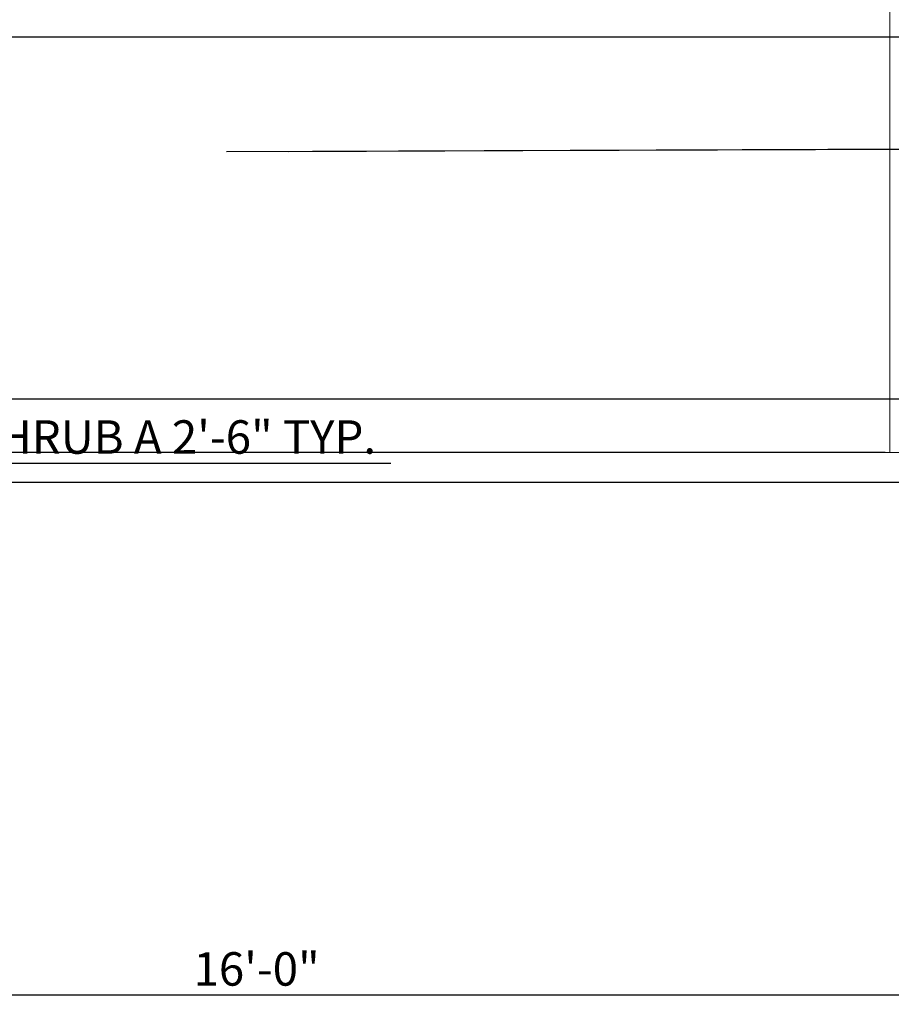
# Model space of a CAD drawing. Units: inches. Extents: x 1239 to 2276906, y 2273 to 321338.
# Tile 2 of 23: x 1424 to 1541, y 2276 to 2408. Entities that reach past the tile are written whole.
import ezdxf

# ---------------------------------------------------------------- set-up
doc = ezdxf.new("R2010")
doc.units = ezdxf.units.IN
for name, color, linetype, lineweight in [('A-ANNO-DIMS', 2, 'Continuous', 18), ('C-PROP', 7, 'Continuous', 25), ('L-PLNT', 94, 'Continuous', 13)]:
    doc.layers.add(name, color=color, linetype=linetype, lineweight=lineweight)
doc.styles.get("Standard").update_dxf_attribs({"font": 'arial.ttf'})
doc.dimstyles.new('ISO-25', dxfattribs={"dimtxt": 4.5, "dimasz": 4, "dimexe": 1.25, "dimexo": 0.625, "dimtad": 1, "dimdec": 1, "dimlunit": 3, "dimtxsty": 'Standard', "dimcen": 2.5, "dimadec": 0, "dimazin": 0, "dimtfac": 1, "dimtdec": 1, "dimtmove": 0, "dimatfit": 3, "dimfxl": 1, "dimarcsym": 0})

# ---------------------------------------------------------------- blocks, each defined once
blk = doc.blocks.new('*D76')
at = {"layer": 'A-ANNO-DIMS', "color": 0, "lineweight": -2, "transparency": 16777216}
for p, q in [((1381.23, 2352.31), (1381.23, 2347.21)), ((1411.06, 2352.31), (1411.06, 2347.21)), ((1385.23, 2348.46), (1407.06, 2348.46)), ((1411.06, 2348.46), (1473.41, 2348.46))]:
    blk.add_line(p, q, dxfattribs=at)
at = {"layer": 'A-ANNO-DIMS', "color": 0, "transparency": 16777216}
for points in [[(1385.23, 2349.13), (1385.23, 2347.79), (1381.23, 2348.46)], [(1407.06, 2349.13), (1407.06, 2347.79), (1411.06, 2348.46)]]:
    blk.add_solid(points, dxfattribs=at)
at = {"layer": 'Defpoints', "color": 0, "transparency": 16777216}
for p in [(1381.23, 2352.93), (1411.06, 2352.93), (1411.06, 2348.46)]:
    blk.add_point(p, dxfattribs=at)
at = {"layer": 'A-ANNO-DIMS', "color": 0, "transparency": 16777216, "insert": (1444.23, 2351.41), "char_height": 4.5, "attachment_point": 5}
blk.add_mtext('SHRUB A 2\'-6" TYP.', dxfattribs=at)
blk = doc.blocks.new('*D89')
at = {"layer": 'A-ANNO-DIMS', "color": 0, "lineweight": -2, "transparency": 16777216}
for p, q in [((1359.38, 3215.77), (1359.38, 2275.7)), ((1551.38, 3215.77), (1551.38, 2275.7)), ((1363.38, 2276.95), (1547.38, 2276.95))]:
    blk.add_line(p, q, dxfattribs=at)
at = {"layer": 'A-ANNO-DIMS', "color": 0, "transparency": 16777216}
for points in [[(1363.38, 2277.61), (1363.38, 2276.28), (1359.38, 2276.95)], [(1547.38, 2277.61), (1547.38, 2276.28), (1551.38, 2276.95)]]:
    blk.add_solid(points, dxfattribs=at)
at = {"layer": 'Defpoints', "color": 0, "transparency": 16777216}
for p in [(1359.38, 3216.4), (1551.38, 3216.4), (1551.38, 2276.95)]:
    blk.add_point(p, dxfattribs=at)
at = {"layer": 'A-ANNO-DIMS', "color": 0, "transparency": 16777216, "insert": (1455.38, 2279.87), "char_height": 4.5, "attachment_point": 5}
blk.add_mtext('16\'-0"', dxfattribs=at)
blk = doc.blocks.new('*D103')
at = {"layer": 'A-ANNO-DIMS', "color": 0, "lineweight": -2, "transparency": 16777216}
for p, q in [((1539.93, 2607.52), (1247.33, 2607.52)), ((1248.58, 2353.9), (1248.58, 2603.52)), ((1539.93, 2349.9), (1247.33, 2349.9))]:
    blk.add_line(p, q, dxfattribs=at)
at = {"layer": 'A-ANNO-DIMS', "color": 0, "transparency": 16777216}
for points in [[(1247.92, 2603.52), (1249.25, 2603.52), (1248.58, 2607.52)], [(1247.92, 2353.9), (1249.25, 2353.9), (1248.58, 2349.9)]]:
    blk.add_solid(points, dxfattribs=at)
at = {"layer": 'Defpoints', "color": 0, "transparency": 16777216}
for p in [(1248.58, 2607.52), (1540.55, 2607.52), (1540.55, 2349.9)]:
    blk.add_point(p, dxfattribs=at)
at = {"layer": 'A-ANNO-DIMS', "color": 0, "transparency": 16777216, "insert": (1245.63, 2478.71), "char_height": 4.5, "attachment_point": 5, "rotation": 90}
blk.add_mtext('21\'-5 1/2"', dxfattribs=at)
blk = doc.blocks.new('*D118')
at = {"layer": 'A-ANNO-DIMS', "color": 0, "lineweight": -2, "transparency": 16777216}
for p, q in [((1745.95, 2405.77), (1247.33, 2405.77)), ((1248.58, 2361.06), (1248.58, 2401.77)), ((1745.95, 2357.06), (1247.33, 2357.06))]:
    blk.add_line(p, q, dxfattribs=at)
at = {"layer": 'A-ANNO-DIMS', "color": 0, "transparency": 16777216}
for points in [[(1247.92, 2401.77), (1249.25, 2401.77), (1248.58, 2405.77)], [(1247.92, 2361.06), (1249.25, 2361.06), (1248.58, 2357.06)]]:
    blk.add_solid(points, dxfattribs=at)
at = {"layer": 'Defpoints', "color": 0, "transparency": 16777216}
for p in [(1248.58, 2405.77), (1746.57, 2405.77), (1746.57, 2357.06)]:
    blk.add_point(p, dxfattribs=at)
at = {"layer": 'A-ANNO-DIMS', "color": 0, "transparency": 16777216, "insert": (1245.63, 2381.42), "char_height": 4.5, "attachment_point": 5, "rotation": 90}
blk.add_mtext('4\'-0 1/2"', dxfattribs=at)
blk = doc.blocks.new('*D119')
at = {"layer": 'A-ANNO-DIMS', "color": 0, "lineweight": -2, "transparency": 16777216}
for p, q in [((1451.32, 2390.4), (1624.69, 2391)), ((1744.46, 2391.42), (1628.69, 2391.01))]:
    blk.add_line(p, q, dxfattribs=at)
at = {"layer": 'A-ANNO-DIMS', "color": 0, "transparency": 16777216}
blk.add_solid([(1628.68, 2391.68), (1628.69, 2390.35), (1624.69, 2391)], dxfattribs=at)
at = {"layer": 'Defpoints', "color": 0, "transparency": 16777216}
for p in [(1451.32, 2390.4), (1624.69, 2391)]:
    blk.add_point(p, dxfattribs=at)
at = {"layer": 'A-ANNO-DIMS', "color": 0, "transparency": 16777216, "insert": (1728.7, 2394.31), "char_height": 4.5, "attachment_point": 5, "rotation": 0.1991}
blk.add_mtext('R14\'-5 1/2"', dxfattribs=at)
blk = doc.blocks.new('*D120')
at = {"layer": 'A-ANNO-DIMS', "color": 0, "lineweight": -2, "transparency": 16777216}
for p, q in [((1451.32, 2390.4), (1620.69, 2391)), ((1738.06, 2391.42), (1624.68, 2391.01))]:
    blk.add_line(p, q, dxfattribs=at)
at = {"layer": 'A-ANNO-DIMS', "color": 0, "transparency": 16777216}
blk.add_solid([(1624.68, 2391.68), (1624.69, 2390.35), (1620.69, 2391)], dxfattribs=at)
at = {"layer": 'Defpoints', "color": 0, "transparency": 16777216}
for p in [(1451.32, 2390.4), (1620.69, 2391)]:
    blk.add_point(p, dxfattribs=at)
at = {"layer": 'A-ANNO-DIMS', "color": 0, "transparency": 16777216, "insert": (1722.3, 2394.31), "char_height": 4.5, "attachment_point": 5, "rotation": 0.2039}
blk.add_mtext('R14\'-1 1/2"', dxfattribs=at)
blk = doc.blocks.new('*D121')
at = {"layer": 'A-ANNO-DIMS', "color": 0, "lineweight": -2, "transparency": 16777216}
for p, q in [((1459.68, 2390.4), (1610.05, 2391)), ((1716.03, 2391.42), (1614.05, 2391.02))]:
    blk.add_line(p, q, dxfattribs=at)
at = {"layer": 'A-ANNO-DIMS', "color": 0, "transparency": 16777216}
blk.add_solid([(1614.05, 2391.68), (1614.06, 2390.35), (1610.05, 2391)], dxfattribs=at)
at = {"layer": 'Defpoints', "color": 0, "transparency": 16777216}
for p in [(1459.68, 2390.4), (1610.05, 2391)]:
    blk.add_point(p, dxfattribs=at)
at = {"layer": 'A-ANNO-DIMS', "color": 0, "transparency": 16777216, "insert": (1700.26, 2394.31), "char_height": 4.5, "attachment_point": 5, "rotation": 0.2296}
blk.add_mtext('R12\'-6 1/2"', dxfattribs=at)

msp = doc.modelspace()

# ---------------------------------------------------------------- linework, layer by layer
at = {"layer": 'C-PROP'}
msp.add_lwpolyline([(1970.38, 2345.9), (1970.38, 3545.9), (1310.38, 3545.9), (1310.38, 2345.9), (1644.79, 2345.9)], dxfattribs=at)
at = {"layer": 'L-PLNT'}
for p, q in [((1540.55, 2607.52), (1540.55, 2349.9)), ((1314.38, 2349.9), (1543.55, 2349.9))]:
    msp.add_line(p, q, dxfattribs=at)

# ---------------------------------------------------------------- dimensions: what is measured, and where the dimension line sits
at = {"layer": 'A-ANNO-DIMS'}
dim = msp.add_linear_dim(base=(1551.38, 2276.95), p1=(1359.38, 3216.4), p2=(1551.38, 3216.4), dimstyle='ISO-25', override={"dimdec": 1, "dimlfac": 1, "dimrnd": 0, "dimzin": 1, "dimdsep": 46, "dimlunit": 4, "dimfrac": 2}, dxfattribs=at)
dim.commit()
dim.dimension.update_dxf_attribs({"geometry": '*D89', "text_midpoint": (1455.38, 2279.87)})
for base, p1, p2, picture, middle in [((1248.58, 2607.52), (1540.55, 2349.9), (1540.55, 2607.52), '*D103', (1245.63, 2478.71)), ((1248.58, 2405.77), (1746.57, 2357.06), (1746.57, 2405.77), '*D118', (1245.63, 2381.42))]:
    dim = msp.add_linear_dim(base=base, p1=p1, p2=p2, angle=90, dimstyle='ISO-25', override={"dimdec": 1, "dimlfac": 1, "dimrnd": 0, "dimzin": 1, "dimdsep": 46, "dimlunit": 4, "dimfrac": 2}, dxfattribs=at)
    dim.commit()
    dim.dimension.update_dxf_attribs({"geometry": picture, "text_midpoint": middle})
for center, mpoint, picture, middle in [((1451.32, 2390.4), (1620.69, 2391), '*D120', (1722.31, 2391.36)), ((1451.32, 2390.4), (1624.69, 2391), '*D119', (1728.71, 2391.36)), ((1459.68, 2390.4), (1610.05, 2391), '*D121', (1700.28, 2391.36))]:
    dim = msp.add_radius_dim(center=center, mpoint=mpoint, dimstyle='ISO-25', override={"dimdec": 1, "dimlfac": 1, "dimrnd": 0, "dimzin": 1, "dimdsep": 46, "dimlunit": 4, "dimfrac": 2}, dxfattribs=at)
    dim.commit()
    dim.dimension.update_dxf_attribs({"geometry": picture, "text_midpoint": middle, "dimtype": 164})
dim = msp.add_linear_dim(base=(1411.06, 2348.46), p1=(1381.23, 2352.93), p2=(1411.06, 2352.93), text='SHRUB A <> TYP.', dimstyle='ISO-25', override={"dimdec": 1, "dimlfac": 1, "dimrnd": 0, "dimzin": 1, "dimdsep": 46, "dimlunit": 4, "dimfrac": 2}, dxfattribs=at)
dim.commit()
dim.dimension.update_dxf_attribs({"geometry": '*D76', "text_midpoint": (1444.23, 2351.41)})

doc.saveas('drawing.dxf')
